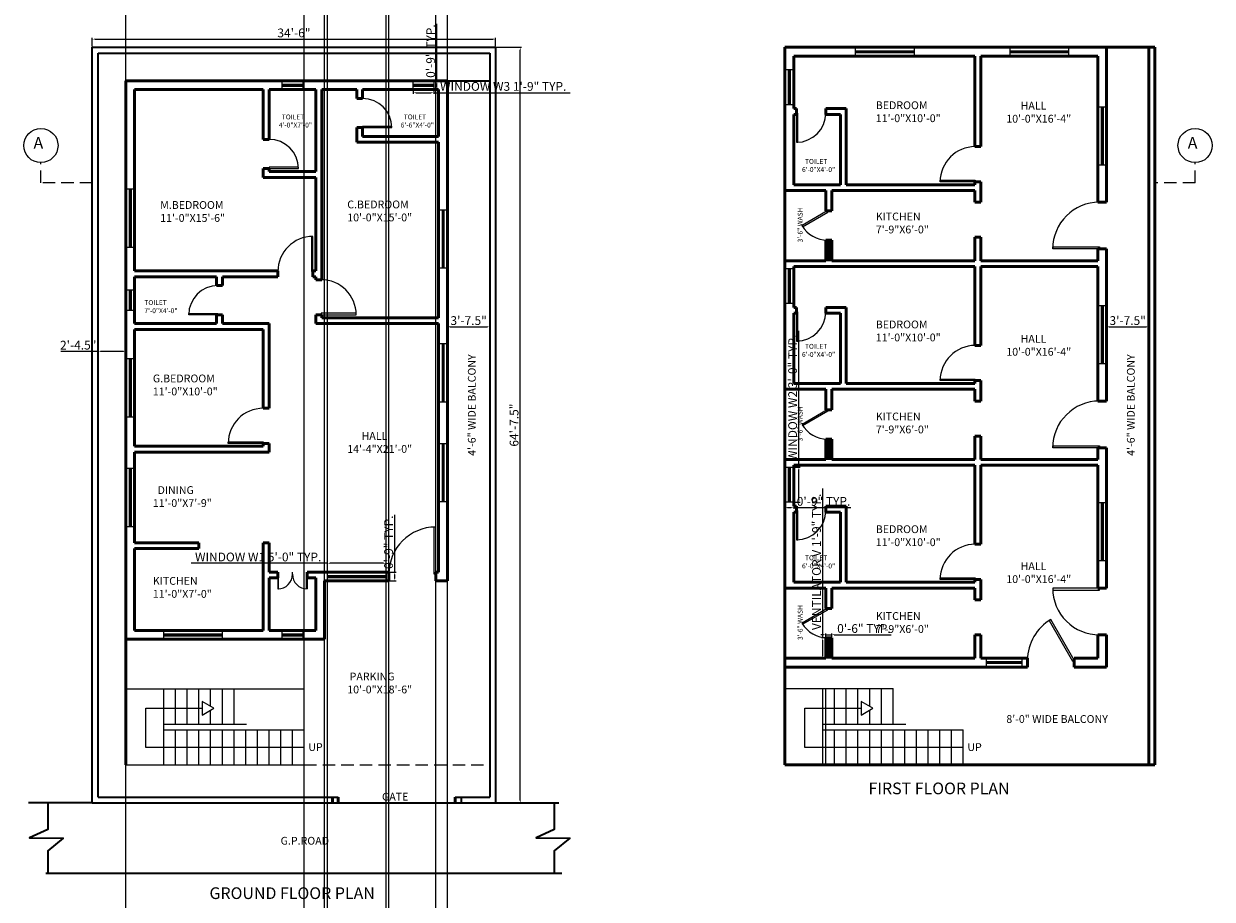
# Model space of a CAD drawing. Units: inches. Extents: x 57 to 1276, y 38 to 1417.
# Tile 1 of 2: x 57 to 1276, y 38 to 936. Entities that reach past the tile are written whole.
import ezdxf

# ---------------------------------------------------------------- set-up
doc = ezdxf.new("R2010")
doc.units = ezdxf.units.IN
doc.linetypes.add('DASHED', pattern=[19.05, 12.7, -6.35])
for name, color, linetype, lineweight in [('A-ANNO-DIMS', 2, 'Continuous', 18), ('A-ANNO-SECT', 1, 'DASHED', 18), ('A-ANNO-SYMB', 1, 'Continuous', 18), ('A-ANNO-TEXT', 7, 'Continuous', 18), ('A-AREA-IDEN', 3, 'Continuous', 18), ('A-CONS', 9, 'Continuous', 13), ('A-DOOR', 3, 'Continuous', 25), ('A-FLOR-OVHD', 8, 'DASHED', 18), ('A-FLOR-STRS', 6, 'Continuous', 25), ('A-GLAZ', 4, 'Continuous', 25), ('A-WALL', 7, 'Continuous', 50), ('C-PROP', 30, 'Continuous', 35)]:
    doc.layers.add(name, color=color, linetype=linetype, lineweight=lineweight)
doc.styles.get("Standard").update_dxf_attribs({"font": 'arial.ttf'})
doc.dimstyles.new('ISO-25', dxfattribs={"dimtxt": 9, "dimasz": 2.5, "dimexe": 1.25, "dimexo": 0.625, "dimtad": 1, "dimlunit": 3, "dimtxsty": 'Standard', "dimcen": 2.5, "dimadec": 0, "dimazin": 0, "dimtfac": 1, "dimtmove": 0, "dimatfit": 3, "dimfxl": 1, "dimarcsym": 0})

# ---------------------------------------------------------------- blocks, each defined once
blk = doc.blocks.new('*U2')
for p, q in [((0, 0), (0, -6)), ((-40, 0), (-40, -6))]:
    blk.add_line(p, q)
blk.add_lwpolyline([(0, 0), (0, 40), (-1.75, 40), (-1.75, 0)], close=True)
blk.add_arc((0, 0), 40, 90, 180)
blk = doc.blocks.new('*U3')
for p, q in [((-40, 0), (-40, 6)), ((0, 0), (0, 6))]:
    blk.add_line(p, q)
blk.add_lwpolyline([(0, 0), (0, -40), (-1.75, -40), (-1.75, 0)], close=True)
blk.add_arc((0, 0), 40, 180, 270)
blk = doc.blocks.new('*U4')
for p, q in [((0, 0), (0, 6)), ((40, 0), (40, 6))]:
    blk.add_line(p, q)
blk.add_lwpolyline([(0, 0), (0, -40), (1.75, -40), (1.75, 0)], close=True)
blk.add_arc((0, 0), 40, 270, 360)
blk = doc.blocks.new('*U5')
for p, q in [((0, 0), (0, 6)), ((40, 0), (40, 6))]:
    blk.add_line(p, q)
blk.add_lwpolyline([(0, 0), (0, -40), (1.75, -40), (1.75, 0)], close=True)
blk.add_arc((0, 0), 40, 270, 0)
blk = doc.blocks.new('*U6')
for p, q in [((0, 0), (0, -6)), ((40, 0), (40, -6))]:
    blk.add_line(p, q)
blk.add_lwpolyline([(0, 0), (0, 40), (1.75, 40), (1.75, 0)], close=True)
blk.add_arc((0, 0), 40, 0, 90)
blk = doc.blocks.new('*D7')
at = {"layer": 'A-ANNO-DIMS', "color": 0, "lineweight": -2, "transparency": 16777216}
for p, q in [((133, 599.8), (94.7, 599.8)), ((133, 608.6), (133, 598.6)), ((159, 599.8), (135.5, 599.8)), ((161.5, 608.6), (161.5, 598.6))]:
    blk.add_line(p, q, dxfattribs=at)
at = {"layer": 'A-ANNO-DIMS', "color": 0, "transparency": 16777216}
for points in [[(135.5, 600.2), (135.5, 599.4), (133, 599.8)], [(159, 600.2), (159, 599.4), (161.5, 599.8)]]:
    blk.add_solid(points, dxfattribs=at)
at = {"layer": 'Defpoints', "color": 0, "transparency": 16777216}
for p in [(133, 609.2), (133, 599.8), (161.5, 609.2)]:
    blk.add_point(p, dxfattribs=at)
at = {"layer": 'A-ANNO-DIMS', "color": 0, "transparency": 16777216, "insert": (112.6, 605.1), "char_height": 9, "width": 37.073, "attachment_point": 5}
blk.add_mtext('2\'-4.5"', dxfattribs=at)
blk = doc.blocks.new('*D8')
at = {"layer": 'A-ANNO-DIMS', "color": 0, "lineweight": -2, "transparency": 16777216}
for p, q in [((491.5, 637.4), (491.5, 623.8)), ((535, 637.4), (535, 623.8)), ((494, 625.1), (532.5, 625.1))]:
    blk.add_line(p, q, dxfattribs=at)
at = {"layer": 'A-ANNO-DIMS', "color": 0, "transparency": 16777216}
for points in [[(494, 625.5), (494, 624.7), (491.5, 625.1)], [(532.5, 625.5), (532.5, 624.7), (535, 625.1)]]:
    blk.add_solid(points, dxfattribs=at)
at = {"layer": 'Defpoints', "color": 0, "transparency": 16777216}
for p in [(491.5, 638), (535, 638), (535, 625.1)]:
    blk.add_point(p, dxfattribs=at)
at = {"layer": 'A-ANNO-DIMS', "color": 0, "transparency": 16777216, "insert": (513.3, 630.3), "char_height": 9, "attachment_point": 5}
blk.add_mtext('3\'-7.5"', dxfattribs=at)
blk = doc.blocks.new('*D9')
at = {"layer": 'A-ANNO-DIMS', "color": 0, "lineweight": -2, "transparency": 16777216}
for p, q in [((127, 912.6), (127, 921.5)), ((129.5, 920.3), (538.5, 920.3)), ((541, 912.6), (541, 921.5))]:
    blk.add_line(p, q, dxfattribs=at)
at = {"layer": 'A-ANNO-DIMS', "color": 0, "transparency": 16777216}
for points in [[(129.5, 920.7), (129.5, 919.9), (127, 920.3)], [(538.5, 920.7), (538.5, 919.9), (541, 920.3)]]:
    blk.add_solid(points, dxfattribs=at)
at = {"layer": 'Defpoints', "color": 0, "transparency": 16777216}
for p in [(541, 920.3), (127, 911.9), (541, 911.9)]:
    blk.add_point(p, dxfattribs=at)
at = {"layer": 'A-ANNO-DIMS', "color": 0, "transparency": 16777216, "insert": (334, 925.5), "char_height": 9, "attachment_point": 5}
blk.add_mtext('34\'-6"', dxfattribs=at)
blk = doc.blocks.new('*D10')
at = {"layer": 'A-ANNO-DIMS', "color": 0, "lineweight": -2, "transparency": 16777216}
for p, q in [((541.6, 911.9), (567.5, 911.9)), ((566.3, 138.9), (566.3, 909.4)), ((541.6, 136.4), (567.5, 136.4))]:
    blk.add_line(p, q, dxfattribs=at)
at = {"layer": 'A-ANNO-DIMS', "color": 0, "transparency": 16777216}
for points in [[(565.9, 909.4), (566.7, 909.4), (566.3, 911.9)], [(565.9, 138.9), (566.7, 138.9), (566.3, 136.4)]]:
    blk.add_solid(points, dxfattribs=at)
at = {"layer": 'Defpoints', "color": 0, "transparency": 16777216}
for p in [(541, 911.9), (566.3, 911.9), (541, 136.4)]:
    blk.add_point(p, dxfattribs=at)
at = {"layer": 'A-ANNO-DIMS', "color": 0, "transparency": 16777216, "insert": (561.1, 524.2), "char_height": 9, "attachment_point": 5, "rotation": 90}
blk.add_mtext('64\'-7.5"', dxfattribs=at)
blk = doc.blocks.new('*D12')
at = {"layer": 'A-ANNO-DIMS', "color": 0, "lineweight": -2, "transparency": 16777216}
for p, q in [((1167.9, 637.4), (1167.9, 623.8)), ((1211.4, 637.4), (1211.4, 623.8)), ((1170.4, 625.1), (1208.9, 625.1))]:
    blk.add_line(p, q, dxfattribs=at)
at = {"layer": 'A-ANNO-DIMS', "color": 0, "transparency": 16777216}
for points in [[(1170.4, 625.5), (1170.4, 624.7), (1167.9, 625.1)], [(1208.9, 625.5), (1208.9, 624.7), (1211.4, 625.1)]]:
    blk.add_solid(points, dxfattribs=at)
at = {"layer": 'Defpoints', "color": 0, "transparency": 16777216}
for p in [(1167.9, 638), (1211.4, 638), (1211.4, 625.1)]:
    blk.add_point(p, dxfattribs=at)
at = {"layer": 'A-ANNO-DIMS', "color": 0, "transparency": 16777216, "insert": (1189.7, 630.3), "char_height": 9, "attachment_point": 5}
blk.add_mtext('3\'-7.5"', dxfattribs=at)
blk = doc.blocks.new('*U13')
for p, q in [((0, 0), (0, 6)), ((40, 0), (40, 6))]:
    blk.add_line(p, q)
blk.add_lwpolyline([(0, 0), (20, -34.6), (21.5, -33.8), (1.5, 0.9)], close=True)
blk.add_arc((0, 0), 40, 300, 360)
blk = doc.blocks.new('*U14')
for p, q in [((-40, 0), (-40, 6)), ((0, 0), (0, 6))]:
    blk.add_line(p, q)
blk.add_lwpolyline([(0, 0), (0, -40), (-1.75, -40), (-1.75, 0)], close=True)
blk.add_arc((0, 0), 40, 180, 270)
blk = doc.blocks.new('*U15')
for p, q in [((0, 0), (0, -6)), ((-40, 0), (-40, -6))]:
    blk.add_line(p, q)
blk.add_lwpolyline([(0, 0), (-20, 34.6), (-21.5, 33.8), (-1.5, -0.9)], close=True)
blk.add_arc((0, 0), 40, 120, 180)
blk = doc.blocks.new('WIN-1500')
for p, q in [((486, 607.9), (486, 547.9)), ((487, 607.9), (487, 547.9)), ((488, 607.9), (488, 547.9))]:
    blk.add_line(p, q)
blk.add_lwpolyline([(491.5, 607.9), (491.5, 547.9), (482.5, 547.9), (482.5, 607.9)], close=True)
blk = doc.blocks.new('WIN-900')
for p, q in [((841.4, 481), (841.4, 445)), ((842.4, 481), (842.4, 445)), ((843.4, 481), (843.4, 445))]:
    blk.add_line(p, q)
blk.add_lwpolyline([(837.9, 481), (846.9, 481), (846.9, 445), (837.9, 445)], close=True)
blk = doc.blocks.new('VENT-525')
for p, q in [((881.9, 284.9), (881.9, 305.9)), ((882.9, 284.9), (882.9, 305.9)), ((883.9, 284.9), (883.9, 305.9))]:
    blk.add_line(p, q)
blk.add_lwpolyline([(879.9, 305.9), (885.9, 305.9), (885.9, 284.9), (879.9, 284.9)], close=True)
blk = doc.blocks.new('WIN-525-V')
for p, q in [((456.5, 873.9), (477.5, 873.9)), ((456.5, 872.9), (477.5, 872.9)), ((456.5, 871.9), (477.5, 871.9))]:
    blk.add_line(p, q)
blk.add_lwpolyline([(456.5, 877.4), (477.5, 877.4), (477.5, 868.4), (456.5, 868.4)], close=True)
blk = doc.blocks.new('*D25')
at = {"layer": 'A-ANNO-DIMS', "color": 0, "lineweight": -2, "transparency": 16777216}
for p, q in [((368.5, 382.4), (228.5, 382.4)), ((368.5, 374.1), (368.5, 383.7)), ((426, 382.4), (371, 382.4)), ((428.5, 374.1), (428.5, 383.7))]:
    blk.add_line(p, q, dxfattribs=at)
at = {"layer": 'A-ANNO-DIMS', "color": 0, "transparency": 16777216}
for points in [[(371, 382.8), (371, 382), (368.5, 382.4)], [(426, 382.8), (426, 382), (428.5, 382.4)]]:
    blk.add_solid(points, dxfattribs=at)
at = {"layer": 'Defpoints', "color": 0, "transparency": 16777216}
for p in [(368.5, 382.4), (368.5, 373.4), (428.5, 373.4)]:
    blk.add_point(p, dxfattribs=at)
at = {"layer": 'A-ANNO-DIMS', "color": 0, "transparency": 16777216, "insert": (297.3, 387.7), "char_height": 9, "attachment_point": 5}
blk.add_mtext('WINDOW W1 5\'-0" TYP.', dxfattribs=at)
blk = doc.blocks.new('*D26')
at = {"layer": 'A-ANNO-DIMS', "color": 0, "lineweight": -2, "transparency": 16777216}
for p, q in [((437.5, 373.4), (437.5, 432)), ((429.1, 373.4), (438.8, 373.4)), ((437.5, 366.9), (437.5, 370.9)), ((429.1, 364.4), (438.8, 364.4))]:
    blk.add_line(p, q, dxfattribs=at)
at = {"layer": 'A-ANNO-DIMS', "color": 0, "transparency": 16777216}
for points in [[(437.1, 370.9), (437.9, 370.9), (437.5, 373.4)], [(437.1, 366.9), (437.9, 366.9), (437.5, 364.4)]]:
    blk.add_solid(points, dxfattribs=at)
at = {"layer": 'Defpoints', "color": 0, "transparency": 16777216}
for p in [(428.5, 373.4), (437.5, 373.4), (428.5, 364.4)]:
    blk.add_point(p, dxfattribs=at)
at = {"layer": 'A-ANNO-DIMS', "color": 0, "transparency": 16777216, "insert": (432.3, 404), "char_height": 9, "attachment_point": 5, "rotation": 90}
blk.add_mtext('0\'-9" TYP.', dxfattribs=at)
blk = doc.blocks.new('*D27')
at = {"layer": 'A-ANNO-DIMS', "color": 0, "lineweight": -2, "transparency": 16777216}
for p, q in [((852.3, 481), (852.3, 620.9)), ((847.5, 481), (853.6, 481)), ((852.3, 447.5), (852.3, 478.5)), ((847.5, 445), (853.6, 445))]:
    blk.add_line(p, q, dxfattribs=at)
at = {"layer": 'A-ANNO-DIMS', "color": 0, "transparency": 16777216}
for points in [[(851.9, 478.5), (852.7, 478.5), (852.3, 481)], [(851.9, 447.5), (852.7, 447.5), (852.3, 445)]]:
    blk.add_solid(points, dxfattribs=at)
at = {"layer": 'Defpoints', "color": 0, "transparency": 16777216}
for p in [(846.9, 481), (852.3, 481), (846.9, 445)]:
    blk.add_point(p, dxfattribs=at)
at = {"layer": 'A-ANNO-DIMS', "color": 0, "transparency": 16777216, "insert": (847, 552.2), "char_height": 9, "attachment_point": 5, "rotation": 90}
blk.add_mtext('WINDOW W2 3\'-0" TYP.', dxfattribs=at)
blk = doc.blocks.new('*D28')
at = {"layer": 'A-ANNO-DIMS', "color": 0, "lineweight": -2, "transparency": 16777216}
for p, q in [((837.9, 444.3), (837.9, 438.3)), ((840.4, 439.6), (844.4, 439.6)), ((846.9, 444.3), (846.9, 438.3)), ((846.9, 439.6), (905.5, 439.6))]:
    blk.add_line(p, q, dxfattribs=at)
at = {"layer": 'A-ANNO-DIMS', "color": 0, "transparency": 16777216}
for points in [[(840.4, 440), (840.4, 439.1), (837.9, 439.6)], [(844.4, 440), (844.4, 439.1), (846.9, 439.6)]]:
    blk.add_solid(points, dxfattribs=at)
at = {"layer": 'Defpoints', "color": 0, "transparency": 16777216}
for p in [(837.9, 445), (846.9, 445), (846.9, 439.6)]:
    blk.add_point(p, dxfattribs=at)
at = {"layer": 'A-ANNO-DIMS', "color": 0, "transparency": 16777216, "insert": (877.5, 444.8), "char_height": 9, "attachment_point": 5}
blk.add_mtext('0\'-9" TYP.', dxfattribs=at)
blk = doc.blocks.new('*D29')
at = {"layer": 'A-ANNO-DIMS', "color": 0, "lineweight": -2, "transparency": 16777216}
for p, q in [((456.5, 867.8), (456.5, 864)), ((477.5, 867.8), (477.5, 864)), ((459, 865.3), (475, 865.3)), ((477.5, 865.3), (617.5, 865.3))]:
    blk.add_line(p, q, dxfattribs=at)
at = {"layer": 'A-ANNO-DIMS', "color": 0, "transparency": 16777216}
for points in [[(459, 865.7), (459, 864.9), (456.5, 865.3)], [(475, 865.7), (475, 864.9), (477.5, 865.3)]]:
    blk.add_solid(points, dxfattribs=at)
at = {"layer": 'Defpoints', "color": 0, "transparency": 16777216}
for p in [(456.5, 868.4), (477.5, 868.4), (477.5, 865.3)]:
    blk.add_point(p, dxfattribs=at)
at = {"layer": 'A-ANNO-DIMS', "color": 0, "transparency": 16777216, "insert": (548.8, 870.6), "char_height": 9, "attachment_point": 5}
blk.add_mtext('WINDOW W3 1\'-9" TYP.', dxfattribs=at)
blk = doc.blocks.new('*D30')
at = {"layer": 'A-ANNO-DIMS', "color": 0, "lineweight": -2, "transparency": 16777216}
for p, q in [((480.7, 877.4), (480.7, 936)), ((478.2, 877.4), (481.9, 877.4)), ((478.2, 868.4), (481.9, 868.4)), ((480.7, 870.9), (480.7, 874.9))]:
    blk.add_line(p, q, dxfattribs=at)
at = {"layer": 'A-ANNO-DIMS', "color": 0, "transparency": 16777216}
for points in [[(480.3, 874.9), (481.1, 874.9), (480.7, 877.4)], [(480.3, 870.9), (481.1, 870.9), (480.7, 868.4)]]:
    blk.add_solid(points, dxfattribs=at)
at = {"layer": 'Defpoints', "color": 0, "transparency": 16777216}
for p in [(477.5, 877.4), (477.5, 868.4), (480.7, 877.4)]:
    blk.add_point(p, dxfattribs=at)
at = {"layer": 'A-ANNO-DIMS', "color": 0, "transparency": 16777216, "insert": (475.5, 908), "char_height": 9, "attachment_point": 5, "rotation": 90}
blk.add_mtext('0\'-9" TYP.', dxfattribs=at)
blk = doc.blocks.new('*D31')
at = {"layer": 'A-ANNO-DIMS', "color": 0, "lineweight": -2, "transparency": 16777216}
for p, q in [((876.8, 305.9), (876.8, 459.3)), ((879.3, 305.9), (875.5, 305.9)), ((876.8, 287.4), (876.8, 303.4)), ((879.3, 284.9), (875.5, 284.9))]:
    blk.add_line(p, q, dxfattribs=at)
at = {"layer": 'A-ANNO-DIMS', "color": 0, "transparency": 16777216}
for points in [[(876.3, 303.4), (877.2, 303.4), (876.8, 305.9)], [(876.3, 287.4), (877.2, 287.4), (876.8, 284.9)]]:
    blk.add_solid(points, dxfattribs=at)
at = {"layer": 'Defpoints', "color": 0, "transparency": 16777216}
for p in [(876.8, 305.9), (879.9, 305.9), (879.9, 284.9)]:
    blk.add_point(p, dxfattribs=at)
at = {"layer": 'A-ANNO-DIMS', "color": 0, "transparency": 16777216, "insert": (871.5, 383.9), "char_height": 9, "attachment_point": 5, "rotation": 90}
blk.add_mtext('VENTILATOR V 1\'-9" TYP.', dxfattribs=at)
blk = doc.blocks.new('*D32')
at = {"layer": 'A-ANNO-DIMS', "color": 0, "lineweight": -2, "transparency": 16777216}
for p, q in [((877.4, 309.1), (874.9, 309.1)), ((879.9, 306.6), (879.9, 310.3)), ((879.9, 309.1), (885.9, 309.1)), ((885.9, 306.6), (885.9, 310.3)), ((888.4, 309.1), (947, 309.1))]:
    blk.add_line(p, q, dxfattribs=at)
at = {"layer": 'A-ANNO-DIMS', "color": 0, "transparency": 16777216}
for points in [[(877.4, 309.5), (877.4, 308.7), (879.9, 309.1)], [(888.4, 309.5), (888.4, 308.7), (885.9, 309.1)]]:
    blk.add_solid(points, dxfattribs=at)
at = {"layer": 'Defpoints', "color": 0, "transparency": 16777216}
for p in [(879.9, 305.9), (885.9, 309.1), (885.9, 305.9)]:
    blk.add_point(p, dxfattribs=at)
at = {"layer": 'A-ANNO-DIMS', "color": 0, "transparency": 16777216, "insert": (919, 314.3), "char_height": 9, "attachment_point": 5}
blk.add_mtext('0\'-6" TYP.', dxfattribs=at)

msp = doc.modelspace()

# ---------------------------------------------------------------- linework, layer by layer
at = {"layer": 'A-ANNO-SECT'}
for p, q in [((74.298, 772.811), (74.298, 793.831)), ((1258.891, 772.811), (1258.891, 793.514)), ((127.017, 772.811), (74.298, 772.811)), ((1258.891, 772.811), (1217.41, 772.811))]:
    msp.add_line(p, q, dxfattribs=at)
at = {"layer": 'A-ANNO-SYMB'}
for centre in [(74.298, 811.087), (1258.891, 811.087)]:
    msp.add_circle(centre, 17.573, dxfattribs=at)
at = {"layer": 'A-CONS'}
for p in [(161.517, 877.429), (161.517, 175.429), (344.517, 175.429), (365.517, 304.429), (368.517, 364.429), (428.517, 364.429), (431.517, 368.029), (479.517, 364.429), (491.517, 364.429)]:
    msp.add_xline(p, (0, 1), dxfattribs=at)
at = {"layer": 'A-FLOR-OVHD'}
msp.add_line((344.517, 175.429), (535.017, 175.429), dxfattribs=at)
at = {"layer": 'A-FLOR-STRS'}
for p, q in [((161.517, 253.429), (344.517, 253.429)), ((200.517, 175.429), (200.517, 253.429)), ((212.517, 217.429), (212.517, 253.429)), ((224.517, 217.429), (224.517, 253.429)), ((236.517, 217.429), (236.517, 253.429)), ((248.517, 235.508), (248.517, 253.429)), ((260.517, 217.429), (260.517, 253.429)), ((272.517, 217.429), (272.517, 253.429)), ((837.91, 254.023), (948.91, 254.023)), ((876.91, 175.429), (876.91, 254.023)), ((879.91, 175.429), (879.91, 254.023)), ((888.91, 217.429), (888.91, 254.023)), ((900.91, 217.429), (900.91, 254.023)), ((912.91, 217.429), (912.91, 254.023)), ((924.91, 235.508), (924.91, 254.023)), ((936.91, 217.429), (936.91, 254.023)), ((948.91, 217.429), (948.91, 254.023)), ((182.037, 193.429), (182.037, 233.654)), ((182.037, 233.654), (239.715, 233.654)), ((248.517, 217.429), (248.517, 231.801)), ((858.43, 193.429), (858.43, 233.654)), ((858.43, 233.654), (916.108, 233.654)), ((924.91, 217.429), (924.91, 231.801)), ((200.517, 217.429), (285.472, 217.429)), ((200.517, 211.429), (344.517, 211.429)), ((212.517, 175.429), (212.517, 211.429)), ((224.517, 175.429), (224.517, 211.429)), ((236.517, 175.429), (236.517, 211.429)), ((248.517, 175.429), (248.517, 211.429)), ((260.517, 175.429), (260.517, 211.429)), ((272.517, 175.429), (272.517, 211.429)), ((284.517, 175.429), (284.517, 211.429)), ((296.517, 175.429), (296.517, 211.429)), ((308.517, 175.429), (308.517, 211.429)), ((320.517, 175.429), (320.517, 211.429)), ((332.517, 175.429), (332.517, 211.429)), ((344.517, 175.429), (344.517, 211.429)), ((876.91, 217.429), (961.865, 217.429)), ((876.91, 211.429), (1020.91, 211.429)), ((888.91, 175.429), (888.91, 211.429)), ((900.91, 175.429), (900.91, 211.429)), ((912.91, 175.429), (912.91, 211.429)), ((924.91, 175.429), (924.91, 211.429)), ((936.91, 175.429), (936.91, 211.429)), ((948.91, 175.429), (948.91, 211.429)), ((960.91, 175.429), (960.91, 211.429)), ((972.91, 175.429), (972.91, 211.429)), ((984.91, 175.429), (984.91, 211.429)), ((996.91, 175.429), (996.91, 211.429)), ((1008.91, 175.429), (1008.91, 211.429)), ((1020.91, 175.429), (1020.91, 211.429)), ((344.517, 193.429), (182.037, 193.429)), ((1020.91, 193.429), (858.43, 193.429)), ((161.517, 175.429), (344.517, 175.429))]:
    msp.add_line(p, q, dxfattribs=at)
for points in [[(251.727, 233.654), (239.715, 240.589), (239.715, 226.72)], [(928.119, 233.654), (916.108, 240.589), (916.108, 226.72)]]:
    msp.add_lwpolyline(points, close=True, dxfattribs=at)
at = {"layer": 'A-WALL'}
for p, q in [((837.91, 911.929), (1167.91, 911.929)), ((837.91, 692.929), (837.91, 911.929)), ((846.91, 902.929), (1032.91, 902.929)), ((846.91, 848.929), (846.91, 902.929)), ((1032.91, 809.929), (1032.91, 902.929)), ((1038.91, 902.929), (1158.91, 902.929)), ((1038.91, 809.929), (1038.91, 902.929)), ((1158.91, 752.929), (1158.91, 902.929)), ((1167.91, 911.929), (1217.41, 911.929)), ((1167.91, 752.929), (1167.91, 911.929)), ((1211.41, 911.929), (1211.41, 175.429)), ((1217.41, 911.929), (1217.41, 175.429)), ((161.517, 877.429), (491.517, 877.429)), ((161.517, 175.429), (161.517, 877.429)), ((170.517, 868.429), (302.517, 868.429)), ((170.517, 682.429), (170.517, 868.429)), ((302.517, 817.429), (302.517, 868.429)), ((308.517, 868.429), (356.517, 868.429)), ((308.517, 817.429), (308.517, 868.429)), ((356.517, 784.429), (356.517, 868.429)), ((362.517, 868.429), (398.517, 868.429)), ((362.517, 673.429), (362.517, 868.429)), ((398.517, 859.429), (398.517, 868.429)), ((404.517, 868.429), (482.517, 868.429)), ((404.517, 859.429), (404.517, 868.429)), ((482.517, 820.429), (482.517, 868.429)), ((491.517, 364.429), (491.517, 877.429)), ((404.517, 859.429), (398.517, 859.429)), ((846.91, 848.929), (849.91, 848.929)), ((846.91, 770.929), (846.91, 842.929)), ((846.91, 842.929), (849.91, 842.929)), ((849.91, 848.929), (849.91, 842.929)), ((879.91, 848.929), (879.91, 842.929)), ((879.91, 848.929), (900.91, 848.929)), ((879.91, 842.929), (894.91, 842.929)), ((894.91, 770.929), (894.91, 842.929)), ((900.91, 770.929), (900.91, 848.929)), ((398.517, 814.429), (398.517, 829.429)), ((404.517, 829.429), (398.517, 829.429)), ((404.517, 820.429), (404.517, 829.429)), ((308.517, 817.429), (302.517, 817.429)), ((404.517, 820.429), (482.517, 820.429)), ((398.517, 814.429), (482.517, 814.429)), ((482.517, 634.429), (482.517, 814.429)), ((1032.91, 809.929), (1038.91, 809.929)), ((302.517, 778.429), (302.517, 787.429)), ((308.517, 787.429), (302.517, 787.429)), ((308.517, 784.429), (308.517, 787.429)), ((308.517, 784.429), (356.517, 784.429)), ((302.517, 778.429), (356.517, 778.429)), ((356.517, 682.429), (356.517, 778.429)), ((846.91, 770.929), (894.91, 770.929)), ((900.91, 770.929), (1032.91, 770.929)), ((1032.91, 770.929), (1032.91, 773.929)), ((1032.91, 773.929), (1038.91, 773.929)), ((1038.91, 752.929), (1038.91, 773.929)), ((837.91, 764.929), (879.91, 764.929)), ((879.91, 743.929), (879.91, 764.929)), ((885.91, 764.929), (1032.91, 764.929)), ((885.91, 743.929), (885.91, 764.929)), ((1032.91, 752.929), (1032.91, 764.929)), ((1032.91, 752.929), (1038.91, 752.929)), ((1158.91, 752.929), (1167.91, 752.929)), ((885.91, 743.929), (879.91, 743.929)), ((879.91, 692.929), (879.91, 713.929)), ((885.91, 713.929), (879.91, 713.929)), ((885.91, 692.929), (885.91, 713.929)), ((1032.91, 692.929), (1032.91, 716.929)), ((1032.91, 716.929), (1038.91, 716.929)), ((1038.91, 692.929), (1038.91, 716.929)), ((1158.91, 692.929), (1158.91, 704.929)), ((1158.91, 704.929), (1167.91, 704.929)), ((1167.91, 548.929), (1167.91, 704.929)), ((837.91, 175.429), (837.91, 692.929)), ((837.91, 692.929), (879.91, 692.929)), ((846.91, 686.929), (1032.91, 686.929)), ((846.91, 644.929), (846.91, 686.929)), ((885.91, 692.929), (1032.91, 692.929)), ((1032.91, 605.929), (1032.91, 686.929)), ((1038.91, 692.929), (1158.91, 692.929)), ((1038.91, 686.929), (1158.91, 686.929)), ((1038.91, 605.929), (1038.91, 686.929)), ((1158.91, 548.929), (1158.91, 686.929)), ((170.517, 682.429), (317.517, 682.429)), ((170.517, 676.429), (254.517, 676.429)), ((170.517, 628.429), (170.517, 676.429)), ((254.517, 667.429), (254.517, 676.429)), ((260.517, 676.429), (317.517, 676.429)), ((260.517, 667.429), (260.517, 676.429)), ((317.517, 676.429), (317.517, 682.429)), ((353.517, 676.429), (353.517, 682.429)), ((353.517, 682.429), (356.517, 682.429)), ((353.517, 676.429), (356.517, 676.429)), ((356.517, 673.429), (356.517, 676.429)), ((362.517, 673.429), (356.517, 673.429)), ((260.517, 667.429), (254.517, 667.429)), ((254.517, 628.429), (254.517, 637.429)), ((260.517, 637.429), (254.517, 637.429)), ((260.517, 628.429), (260.517, 637.429)), ((356.517, 628.429), (356.517, 637.429)), ((362.517, 637.429), (356.517, 637.429)), ((362.517, 634.429), (362.517, 637.429)), ((362.517, 634.429), (482.517, 634.429)), ((846.91, 644.929), (849.91, 644.929)), ((846.91, 566.929), (846.91, 638.929)), ((846.91, 638.929), (849.91, 638.929)), ((849.91, 638.929), (849.91, 644.929)), ((879.91, 638.929), (879.91, 644.929)), ((879.91, 644.929), (900.91, 644.929)), ((879.91, 638.929), (894.91, 638.929)), ((894.91, 566.929), (894.91, 638.929)), ((900.91, 566.929), (900.91, 644.929)), ((170.517, 628.429), (254.517, 628.429)), ((170.517, 622.429), (302.517, 622.429)), ((170.517, 502.429), (170.517, 622.429)), ((260.517, 628.429), (308.517, 628.429)), ((302.517, 541.429), (302.517, 622.429)), ((308.517, 541.429), (308.517, 628.429)), ((356.517, 628.429), (482.517, 628.429)), ((482.517, 373.429), (482.517, 628.429)), ((1032.91, 605.929), (1038.91, 605.929)), ((846.91, 566.929), (894.91, 566.929)), ((900.91, 566.929), (1032.91, 566.929)), ((1032.91, 566.929), (1032.91, 569.929)), ((1032.91, 569.929), (1038.91, 569.929)), ((1038.91, 548.929), (1038.91, 569.929)), ((837.91, 560.929), (879.91, 560.929)), ((879.91, 539.929), (879.91, 560.929)), ((885.91, 560.929), (1032.91, 560.929)), ((885.91, 539.929), (885.91, 560.929)), ((1032.91, 548.929), (1032.91, 560.929)), ((1032.91, 548.929), (1038.91, 548.929)), ((1158.91, 548.929), (1167.91, 548.929)), ((302.517, 541.429), (308.517, 541.429)), ((885.91, 539.929), (879.91, 539.929)), ((1032.91, 488.929), (1032.91, 512.929)), ((1032.91, 512.929), (1038.91, 512.929)), ((1038.91, 488.929), (1038.91, 512.929)), ((170.517, 502.429), (302.517, 502.429)), ((302.517, 502.429), (302.517, 505.429)), ((302.517, 505.429), (308.517, 505.429)), ((308.517, 496.429), (308.517, 505.429)), ((879.91, 488.929), (879.91, 509.929)), ((885.91, 509.929), (879.91, 509.929)), ((885.91, 488.929), (885.91, 509.929)), ((1158.91, 488.929), (1158.91, 500.929)), ((1158.91, 500.929), (1167.91, 500.929)), ((1167.91, 356.929), (1167.91, 500.929)), ((170.517, 496.429), (308.517, 496.429)), ((170.517, 403.429), (170.517, 496.429)), ((837.91, 488.929), (879.91, 488.929)), ((885.91, 488.929), (1032.91, 488.929)), ((1038.91, 488.929), (1158.91, 488.929)), ((846.91, 482.929), (1032.91, 482.929)), ((846.91, 440.929), (846.91, 482.929)), ((1032.91, 401.929), (1032.91, 482.929)), ((1038.91, 482.929), (1158.91, 482.929)), ((1038.91, 401.929), (1038.91, 482.929)), ((1158.91, 356.929), (1158.91, 482.929)), ((846.91, 440.929), (849.91, 440.929)), ((849.91, 434.929), (849.91, 440.929)), ((879.91, 434.929), (879.91, 440.929)), ((879.91, 440.929), (900.91, 440.929)), ((900.91, 362.929), (900.91, 440.929)), ((846.91, 362.929), (846.91, 434.929)), ((846.91, 434.929), (849.91, 434.929)), ((879.91, 434.929), (894.91, 434.929)), ((894.91, 362.929), (894.91, 434.929)), ((170.517, 403.429), (236.517, 403.429)), ((236.517, 397.429), (236.517, 403.429)), ((302.517, 313.429), (302.517, 403.429)), ((302.517, 403.429), (308.517, 403.429)), ((308.517, 373.429), (308.517, 403.429)), ((170.517, 313.429), (170.517, 397.429)), ((170.517, 397.429), (236.517, 397.429)), ((1032.91, 401.929), (1038.91, 401.929)), ((308.517, 373.429), (317.517, 373.429)), ((308.517, 313.429), (308.517, 367.429)), ((308.517, 367.429), (317.517, 367.429)), ((317.517, 367.429), (317.517, 373.429)), ((347.517, 367.429), (347.517, 373.429)), ((347.517, 373.429), (431.517, 373.429)), ((347.517, 367.429), (356.517, 367.429)), ((356.517, 313.429), (356.517, 367.429)), ((431.517, 373.429), (431.517, 364.429)), ((479.517, 373.429), (479.517, 364.429)), ((479.517, 373.429), (482.517, 373.429)), ((1032.91, 362.929), (1032.91, 365.929)), ((1032.91, 365.929), (1038.91, 365.929)), ((1038.91, 344.929), (1038.91, 365.929)), ((365.517, 304.429), (365.517, 364.429)), ((365.517, 364.429), (431.517, 364.429)), ((479.517, 364.429), (491.517, 364.429)), ((837.91, 356.929), (879.91, 356.929)), ((846.91, 362.929), (894.91, 362.929)), ((879.91, 335.929), (879.91, 356.929)), ((885.91, 356.929), (1032.91, 356.929)), ((885.91, 335.929), (885.91, 356.929)), ((900.91, 362.929), (1032.91, 362.929)), ((1032.91, 344.929), (1032.91, 356.929)), ((1158.91, 356.929), (1167.91, 356.929)), ((1032.91, 344.929), (1038.91, 344.929)), ((879.91, 335.929), (885.91, 335.929)), ((170.517, 313.429), (302.517, 313.429)), ((308.517, 313.429), (356.517, 313.429)), ((879.91, 284.929), (879.91, 305.929)), ((879.91, 305.929), (885.91, 305.929)), ((885.91, 284.929), (885.91, 305.929)), ((1032.91, 284.929), (1032.91, 308.929)), ((1032.91, 308.929), (1038.91, 308.929)), ((1038.91, 284.929), (1038.91, 308.929)), ((1158.91, 284.929), (1158.91, 308.929)), ((1158.91, 308.929), (1167.91, 308.929)), ((1167.91, 275.929), (1167.91, 308.929)), ((161.517, 175.429), (161.517, 304.429)), ((161.517, 304.429), (365.517, 304.429)), ((837.91, 284.929), (879.91, 284.929)), ((885.91, 284.929), (1032.91, 284.929)), ((1038.91, 284.929), (1086.91, 284.929)), ((1086.91, 284.929), (1086.91, 275.929)), ((1134.91, 284.929), (1134.91, 275.929)), ((1134.91, 284.929), (1158.91, 284.929)), ((837.91, 275.929), (1086.91, 275.929)), ((1134.91, 275.929), (1167.91, 275.929)), ((837.91, 175.429), (1217.41, 175.429)), ((373.522, 142.429), (373.522, 136.429)), ((379.522, 142.429), (379.522, 136.429)), ((499.522, 142.429), (499.522, 136.429))]:
    msp.add_line(p, q, dxfattribs=at)
at = {"layer": 'C-PROP'}
for p, q in [((127.017, 136.429), (127.017, 911.929)), ((127.017, 911.929), (541.017, 911.929)), ((133.017, 905.929), (535.017, 905.929)), ((133.017, 142.429), (133.017, 905.929)), ((535.017, 905.929), (535.017, 142.429)), ((541.017, 911.929), (541.017, 136.429)), ((491.517, 877.429), (535.017, 877.429)), ((127.017, 136.429), (61.426, 136.429)), ((127.017, 136.429), (541.017, 136.429)), ((133.017, 142.429), (379.522, 142.429)), ((499.522, 142.429), (535.017, 142.429)), ((505.522, 142.429), (505.522, 136.429)), ((541.017, 136.429), (605.721, 136.429)), ((79.306, 64.429), (609.039, 64.429))]:
    msp.add_line(p, q, dxfattribs=at)
for points in [[(81.344, 136.429), (81.344, 109.276), (62.729, 100.554), (97.243, 100.304), (81.344, 87.274), (81.344, 64.429)], [(601.233, 136.429), (601.233, 109.276), (582.617, 100.554), (617.131, 100.304), (601.233, 87.274), (601.233, 64.429)]]:
    msp.add_lwpolyline(points, dxfattribs=at)

# ---------------------------------------------------------------- block references
at = {"layer": 'A-DOOR'}
for name, p, xscale, yscale, zscale, rotation in [('*U5', (404.517, 829.429), 0.75, 0.75, 0.75, 90), ('*U5', (308.517, 787.429), 0.75, 0.75, 0.75, 90), ('*U3', (1033.21, 773.929), 0.9, 0.9, 0.9, 270), ('*U14', (1160.71, 704.929), 1.200000000000001, 1.200000000000001, 1.200000000000001, 269.9999999999999), ('*U15', (881.41, 743.929), 0.75, 0.75, 0.75, 90), ('*U2', (361.917, 637.429), 0.9, 0.9, 0.9, 270), ('*U6', (256.017, 637.429), 0.75, 0.75, 0.75, 90), ('*U3', (1033.21, 569.929), 0.9, 0.9, 0.9, 270), ('*U14', (1160.71, 500.929), 1.200000000000001, 1.200000000000001, 1.200000000000001, 269.9999999999999), ('*U3', (302.517, 505.429), 0.9, 0.9, 0.9, 270), ('*U15', (881.41, 539.929), 0.75, 0.75, 0.75, 90), ('*U4', (479.517, 371.629), 1.200000000000001, 1.200000000000001, 1.200000000000001, 180), ('*U3', (1033.21, 365.929), 0.9, 0.9, 0.9, 270), ('*U4', (1160.71, 356.929), 1.200000000000001, 1.200000000000001, 1.200000000000001, 269.9999999999999), ('*U15', (881.41, 335.929), 0.75, 0.75, 0.75, 90), ('*U13', (1134.91, 283.129), 1.200000000000001, 1.200000000000001, 1.200000000000001, 180)]:
    msp.add_blockref(name, p, dxfattribs=dict(at, xscale=xscale, yscale=yscale, zscale=zscale, rotation=rotation))
for name, p, xscale, yscale, zscale in [('*U5', (849.91, 844.429), 0.75, 0.75, 0.75), ('*U2', (353.517, 681.829), 0.9, 0.9, 0.9), ('*U5', (849.91, 640.429), 0.75, 0.75, 0.75), ('*U5', (849.91, 436.429), 0.75, 0.75, 0.75), ('*U5', (317.517, 371.179), 0.375, 0.375, 0.375), ('*U3', (347.517, 371.179), 0.375, 0.375, 0.375)]:
    msp.add_blockref(name, p, dxfattribs=dict(at, xscale=xscale, yscale=yscale, zscale=zscale))
at = {"layer": 'A-GLAZ'}
for name, p, rotation in [('WIN-1500', (1518.331, 420.412), 89.99999999999991), ('WIN-1500', (1676.934, 420.412), 89.99999999999984), ('WIN-525-V', (-706.912, 1119.475), 270), ('WIN-1500', (976.396, -118.088), 89.99999999999996), ('WIN-1500', (808.386, -178.088), 90), ('WIN-900', (599.953, 1122.838), 269.9999999999999)]:
    msp.add_blockref(name, p, dxfattribs=dict(at, rotation=rotation))
for name, p in [('WIN-900', (0, 408)), ('WIN-525-V', (-134.53, 0)), ('WIN-525-V', (0, 0)), ('WIN-1500', (676.393, 243.03)), ('WIN-1500', (-321, 158.674)), ('WIN-1500', (0, 137.187)), ('VENT-525', (0, 408)), ('WIN-900', (0, 204)), ('WIN-1500', (676.393, 39.093)), ('WIN-1500', (0, 0)), ('WIN-1500', (-321, -15.45)), ('WIN-1500', (0, -102.448)), ('VENT-525', (0, 204)), ('WIN-1500', (-321, -127.95)), ('WIN-900', (0, 0)), ('WIN-1500', (676.393, -162.987)), ('WIN-525-V', (-134.432, -564)), ('VENT-525', (0, 0))]:
    msp.add_blockref(name, p, dxfattribs=at)

# ---------------------------------------------------------------- texts
at = {"layer": 'A-ANNO-SYMB', "char_height": 12, "attachment_point": 1}
for insert in [(66.716, 819.885), (1251.309, 819.885)]:
    msp.add_mtext_dynamic_manual_height_columns('A', width=11.71893, gutter_width=12.5, heights=[0], dxfattribs=dict(at, insert=insert))
at = {"layer": 'A-ANNO-TEXT', "char_height": 8, "attachment_point": 1, "rotation": 90}
for insert in [(512.544, 492.667), (1188.937, 492.667)]:
    msp.add_mtext_dynamic_manual_height_columns('4\'-6" WIDE BALCONY', width=116.14115, gutter_width=12.5, heights=[0], dxfattribs=dict(at, insert=insert))
at = {"layer": 'A-ANNO-TEXT', "attachment_point": 1}
for s, width, insert, char_height in [('8\'-0" WIDE BALCONY', 115.7649, (1065.13, 226.604), 8), ('UP', 15.64407, (348.773, 197.8), 8), ('UP', 15.64407, (1025.166, 197.8), 8), ('GATE', 31.03351, (424.372, 146.9), 8), ('FIRST FLOOR PLAN', 186.40428, (923.705, 157.385), 12), ('G.P.ROAD', 57.48841, (320.324, 101.68), 8), ('GROUND FLOOR PLAN', 186.40428, (247.312, 49.892), 12)]:
    msp.add_mtext_dynamic_manual_height_columns(s, width=width, gutter_width=12.5, heights=[0], dxfattribs=dict(at, insert=insert, char_height=char_height))
at = {"layer": 'A-AREA-IDEN', "attachment_point": 1}
for s, width, insert, char_height in [('BEDROOM\\P11\'-0"X10\'-0"', 65.64311, (931.169, 856.429), 8), ('      HALL\\P10\'-0"X16\'-4"', 60.95005, (1065.13, 855.945), 8), ('  TOILET\\P4\'-0"X7\'-0"', 33.80507, (318.503, 842.929), 5), ('  TOILET\\P6\'-6"X4\'-0"', 33.80507, (443.664, 842.929), 5), ('  TOILET\\P6\'-0"X4\'-0"', 34.03957, (855.454, 797.276), 5), ('M.BEDROOM\\P11\'-0"X15\'-6"', 69.99395, (196.737, 754.095), 8), ('C.BEDROOM\\P10\'-0"X15\'-0"', 69.99395, (388.737, 754.634), 8), ('KITCHEN\\P7\'-9"X6\'-0"', 51.6589, (931.169, 742.25), 8), ('TOILET\\P7\'-0"X4\'-0"', 33.80507, (180.503, 652.429), 5), ('BEDROOM\\P11\'-0"X10\'-0"', 65.64311, (931.169, 631.476), 8), ('      HALL\\P10\'-0"X16\'-4"', 60.95005, (1065.13, 616.777), 8), ('  TOILET\\P6\'-0"X4\'-0"', 34.03957, (855.454, 607.536), 5), ('G.BEDROOM\\P11\'-0"X10\'-0"', 70.44714, (189.19, 576.07), 8), ('KITCHEN\\P7\'-9"X6\'-0"', 51.6589, (931.169, 537.06), 8), ('      HALL\\P14\'-4"X21\'-0"', 60.95005, (388.737, 517.07), 8), ('  DINING\\P11\'-0"X7\'-9"', 55.23209, (189.19, 461.535), 8), ('BEDROOM\\P11\'-0"X10\'-0"', 65.64311, (931.169, 421.376), 8), ('  TOILET\\P6\'-0"X4\'-0"', 34.03957, (855.454, 390.497), 5), ('      HALL\\P10\'-0"X16\'-4"', 60.95005, (1065.13, 383.494), 8), ('KITCHEN\\P11\'-0"X7\'-0"', 55.23209, (189.19, 368.347), 8), ('KITCHEN\\P7\'-9"X6\'-0"', 51.6589, (931.169, 332.273), 8), (' PARKING\\P10\'-0"X18\'-6"', 64.54131, (388.737, 270.224), 8)]:
    msp.add_mtext_dynamic_manual_height_columns(s, width=width, gutter_width=12.5, heights=[0], dxfattribs=dict(at, insert=insert, char_height=char_height))
at = {"layer": 'A-AREA-IDEN', "char_height": 5, "attachment_point": 1, "rotation": 90}
for insert in [(851.066, 711.693), (851.066, 507.693), (851.066, 303.693)]:
    msp.add_mtext_dynamic_manual_height_columns('3\'-6" WASH', width=37.72336, gutter_width=12.5, heights=[0], dxfattribs=dict(at, insert=insert))

# ---------------------------------------------------------------- dimensions: what is measured, and where the dimension line sits
at = {"layer": 'A-ANNO-DIMS'}
for base, p1, p2, picture, middle in [((541.017, 920.293), (127.017, 911.929), (541.017, 911.929), '*D9', (334.017, 925.516)), ((535.017, 625.078), (491.517, 638.042), (535.017, 638.042), '*D8', (513.267, 630.301)), ((1211.41, 625.078), (1167.91, 638.042), (1211.41, 638.042), '*D12', (1189.66, 630.301)), ((133.017, 599.833), (161.517, 609.224), (133.017, 609.224), '*D7', (112.61, 605.053))]:
    dim = msp.add_linear_dim(base=base, p1=p1, p2=p2, dimstyle='ISO-25', override={"dimclrd": 0, "dimclre": 0, "dimclrt": 0}, dxfattribs=at)
    dim.commit()
    dim.dimension.update_dxf_attribs({"geometry": picture, "text_midpoint": middle})
for base, p1, p2, angle, text, picture, middle in [((480.697, 877.429), (477.547, 868.429), (477.547, 877.429), 90, '<> TYP.', '*D30', (475.477, 907.983)), ((852.31, 480.957), (846.91, 444.957), (846.91, 480.957), 90, 'WINDOW W2 <> TYP.', '*D27', (847.025, 552.202)), ((876.76, 305.929), (879.91, 284.929), (879.91, 305.929), 90, 'VENTILATOR V <> TYP.', '*D31', (871.478, 383.875)), ((437.517, 373.429), (428.517, 364.429), (428.517, 373.429), 90, '<> TYP.', '*D26', (432.297, 403.983)), ((368.517, 382.429), (428.517, 373.429), (368.517, 373.429), 180, 'WINDOW W1 <> TYP.', '*D25', (297.272, 387.71))]:
    dim = msp.add_linear_dim(base=base, p1=p1, p2=p2, angle=angle, text=text, dimstyle='ISO-25', override={"dimdec": 1, "dimrnd": 0, "dimzin": 1, "dimlunit": 4, "dimfrac": 2}, dxfattribs=at)
    dim.commit()
    dim.dimension.update_dxf_attribs({"geometry": picture, "text_midpoint": middle})
dim = msp.add_linear_dim(base=(566.283, 911.929), p1=(541.017, 136.429), p2=(541.017, 911.929), angle=90, dimstyle='ISO-25', override={"dimclrd": 0, "dimclre": 0, "dimclrt": 0}, dxfattribs=at)
dim.commit()
dim.dimension.update_dxf_attribs({"geometry": '*D10', "text_midpoint": (561.063, 524.179)})
for base, p1, p2, text, picture, middle in [((477.547, 865.279), (456.547, 868.429), (477.547, 868.429), 'WINDOW W3 <> TYP.', '*D29', (548.792, 870.563)), ((846.91, 439.557), (837.91, 444.957), (846.91, 444.957), '<> TYP.', '*D28', (877.464, 444.777)), ((885.91, 309.079), (879.91, 305.929), (885.91, 305.929), '<> TYP.', '*D32', (918.964, 314.299))]:
    dim = msp.add_linear_dim(base=base, p1=p1, p2=p2, text=text, dimstyle='ISO-25', override={"dimdec": 1, "dimrnd": 0, "dimzin": 1, "dimlunit": 4, "dimfrac": 2}, dxfattribs=at)
    dim.commit()
    dim.dimension.update_dxf_attribs({"geometry": picture, "text_midpoint": middle})

doc.saveas('drawing.dxf')
